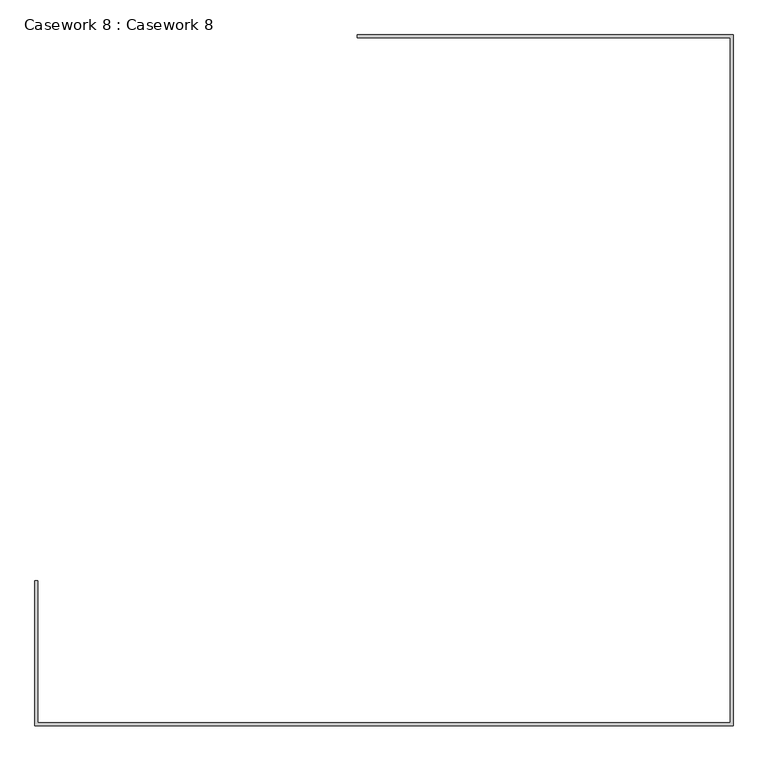
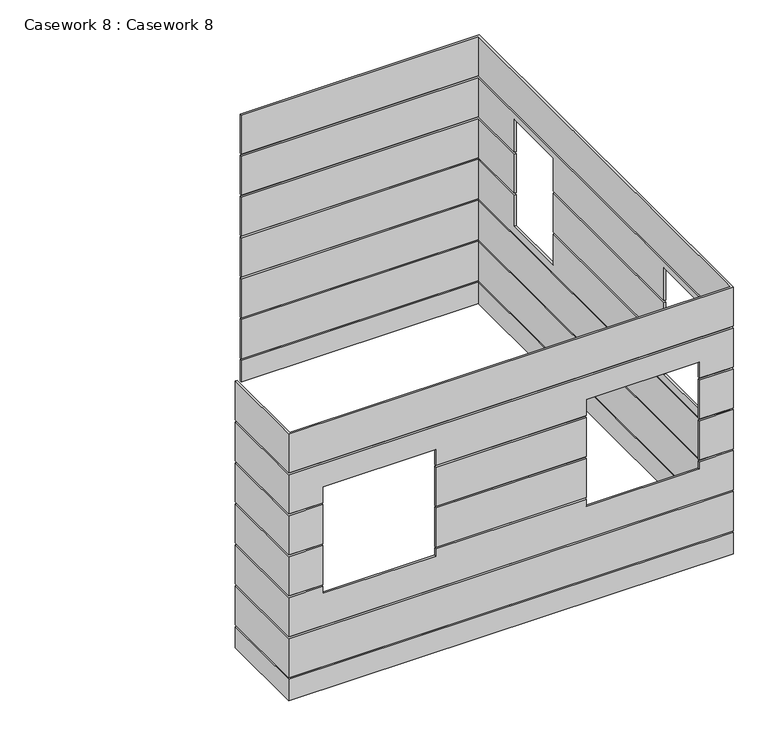
"""IFC4 building model written with IfcOpenShell, lengths in millimetres: furniture geometry, Casework 8 : Casework 8."""

from ifc_helpers import new_model, si_unit, origin, place, context, project, spatial, faceted_brep, source, transform, mapped, element, save


def casework_8_casework_8_de918fe4(model_context):
    return source(origin(), model_context, "Body", "Brep", [
        faceted_brep([(1963.2046034, -9896.6929163, 3750.0), (1988.2046034, -9896.6929163, 3750.0), (1988.2046034, -9896.6929163, 3200.0), (1963.2046034, -9896.6929163, 3200.0), (1963.2046034, -11121.6929163, 3750.0), (7863.2046034, -11121.6929163, 3750.0), (7863.2046034, -5284.1929163, 3750.0), (4688.2046034, -5284.1929163, 3750.0), (4688.2046034, -5309.1929163, 3750.0), (7838.2046034, -5309.1929163, 3750.0), (7838.2046034, -11096.6929163, 3750.0), (1988.2046034, -11096.6929163, 3750.0), (1988.2046034, -11096.6929163, 3200.0), (7838.2046034, -11096.6929163, 3200.0), (7838.2046034, -5309.1929163, 3200.0), (4688.2046034, -5309.1929163, 3200.0), (4688.2046034, -5284.1929163, 3200.0), (7863.2046034, -5284.1929163, 3200.0), (7863.2046034, -11121.6929163, 3200.0), (1963.2046034, -11121.6929163, 3200.0)], [[[0, 1, 2, 3]], [[1, 0, 4, 5, 6, 7, 8, 9, 10, 11]], [[2, 1, 11, 12]], [[3, 2, 12, 13, 14, 15, 16, 17, 18, 19]], [[0, 3, 19, 4]], [[11, 10, 13, 12]], [[5, 4, 19, 18]], [[10, 9, 14, 13]], [[6, 5, 18, 17]], [[8, 7, 16, 15]], [[9, 8, 15, 14]], [[7, 6, 17, 16]]]),
        faceted_brep([(1963.2046034, -9896.6929163, 3175.0), (1988.2046034, -9896.6929163, 3175.0), (1988.2046034, -9896.6929163, 2625.0), (1963.2046034, -9896.6929163, 2625.0), (1963.2046034, -11121.6929163, 3175.0), (7863.2046034, -11121.6929163, 3175.0), (7863.2046034, -5284.1929163, 3175.0), (4688.2046034, -5284.1929163, 3175.0), (4688.2046034, -5309.1929163, 3175.0), (7838.2046034, -5309.1929163, 3175.0), (7838.2046034, -11096.6929163, 3175.0), (1988.2046034, -11096.6929163, 3175.0), (1988.2046034, -11096.6929163, 2625.0), (2413.2046034, -11096.6929163, 2625.0), (2413.2046034, -11121.6929163, 2625.0), (1963.2046034, -11121.6929163, 2625.0), (7838.2046034, -5309.1929163, 2625.0), (4688.2046034, -5309.1929163, 2625.0), (4688.2046034, -5284.1929163, 2625.0), (7863.2046034, -5284.1929163, 2625.0), (7863.2046034, -6134.1929163, 2625.0), (7838.2046034, -6134.1929163, 2625.0), (7413.2046034, -11096.6929163, 2625.0), (7838.2046034, -11096.6929163, 2625.0), (7838.2046034, -10471.6929163, 2625.0), (7863.2046034, -10471.6929163, 2625.0), (7863.2046034, -11121.6929163, 2625.0), (7413.2046034, -11121.6929163, 2625.0), (3913.2046034, -11096.6929163, 2625.0), (5913.2046034, -11096.6929163, 2625.0), (5913.2046034, -11121.6929163, 2625.0), (3913.2046034, -11121.6929163, 2625.0), (7838.2046034, -9571.6929163, 2625.0), (7838.2046034, -7034.1929163, 2625.0), (7863.2046034, -7034.1929163, 2625.0), (7863.2046034, -9571.6929163, 2625.0), (7413.2046034, -11096.6929163, 2850.0), (5913.2046034, -11096.6929163, 2850.0), (3913.2046034, -11096.6929163, 2850.0), (2413.2046034, -11096.6929163, 2850.0), (2413.2046034, -11121.6929163, 2850.0), (3913.2046034, -11121.6929163, 2850.0), (5913.2046034, -11121.6929163, 2850.0), (7413.2046034, -11121.6929163, 2850.0), (7838.2046034, -6134.1929163, 3090.0), (7838.2046034, -7034.1929163, 3090.0), (7838.2046034, -9571.6929163, 3090.0), (7838.2046034, -10471.6929163, 3090.0), (7863.2046034, -10471.6929163, 3090.0), (7863.2046034, -9571.6929163, 3090.0), (7863.2046034, -7034.1929163, 3090.0), (7863.2046034, -6134.1929163, 3090.0)], [[[0, 1, 2, 3]], [[1, 0, 4, 5, 6, 7, 8, 9, 10, 11]], [[2, 1, 11, 12]], [[3, 2, 12, 13, 14, 15]], [[16, 17, 18, 19, 20, 21]], [[22, 23, 24, 25, 26, 27]], [[28, 29, 30, 31]], [[32, 33, 34, 35]], [[0, 3, 15, 4]], [[11, 10, 23, 22, 36, 37, 29, 28, 38, 39, 13, 12]], [[5, 4, 15, 14, 40, 41, 31, 30, 42, 43, 27, 26]], [[10, 9, 16, 21, 44, 45, 33, 32, 46, 47, 24, 23]], [[6, 5, 26, 25, 48, 49, 35, 34, 50, 51, 20, 19]], [[8, 7, 18, 17]], [[9, 8, 17, 16]], [[7, 6, 19, 18]], [[43, 36, 22, 27]], [[37, 42, 30, 29]], [[36, 43, 42, 37]], [[41, 38, 28, 31]], [[39, 40, 14, 13]], [[38, 41, 40, 39]], [[49, 46, 32, 35]], [[47, 48, 25, 24]], [[46, 49, 48, 47]], [[51, 44, 21, 20]], [[45, 50, 34, 33]], [[44, 51, 50, 45]]]),
        faceted_brep([(1963.2046034, -9896.6929163, 2600.0), (1988.2046034, -9896.6929163, 2600.0), (1988.2046034, -9896.6929163, 2050.0), (1963.2046034, -9896.6929163, 2050.0), (1963.2046034, -11121.6929163, 2600.0), (2413.2046034, -11121.6929163, 2600.0), (2413.2046034, -11096.6929163, 2600.0), (1988.2046034, -11096.6929163, 2600.0), (1988.2046034, -11096.6929163, 2050.0), (2413.2046034, -11096.6929163, 2050.0), (2413.2046034, -11121.6929163, 2050.0), (1963.2046034, -11121.6929163, 2050.0)], [[[0, 1, 2, 3]], [[1, 0, 4, 5, 6, 7]], [[2, 1, 7, 8]], [[3, 2, 8, 9, 10, 11]], [[0, 3, 11, 4]], [[8, 7, 6, 9]], [[4, 11, 10, 5]], [[6, 5, 10, 9]]]),
        faceted_brep([(1963.2046034, -9896.6929163, 2025.0), (1988.2046034, -9896.6929163, 2025.0), (1988.2046034, -9896.6929163, 1475.0), (1963.2046034, -9896.6929163, 1475.0), (1963.2046034, -11121.6929163, 2025.0), (2413.2046034, -11121.6929163, 2025.0), (2413.2046034, -11096.6929163, 2025.0), (1988.2046034, -11096.6929163, 2025.0), (1988.2046034, -11096.6929163, 1475.0), (2413.2046034, -11096.6929163, 1475.0), (2413.2046034, -11121.6929163, 1475.0), (1963.2046034, -11121.6929163, 1475.0)], [[[0, 1, 2, 3]], [[1, 0, 4, 5, 6, 7]], [[2, 1, 7, 8]], [[3, 2, 8, 9, 10, 11]], [[0, 3, 11, 4]], [[8, 7, 6, 9]], [[4, 11, 10, 5]], [[6, 5, 10, 9]]]),
        faceted_brep([(1963.2046034, -9896.6929163, 1450.0), (1988.2046034, -9896.6929163, 1450.0), (1988.2046034, -9896.6929163, 900.0), (1963.2046034, -9896.6929163, 900.0), (1963.2046034, -11121.6929163, 1450.0), (2413.2046034, -11121.6929163, 1450.0), (2413.2046034, -11096.6929163, 1450.0), (1988.2046034, -11096.6929163, 1450.0), (7863.2046034, -11121.6929163, 1450.0), (7863.2046034, -5284.1929163, 1450.0), (4688.2046034, -5284.1929163, 1450.0), (4688.2046034, -5309.1929163, 1450.0), (7838.2046034, -5309.1929163, 1450.0), (7838.2046034, -11096.6929163, 1450.0), (7413.2046034, -11096.6929163, 1450.0), (7413.2046034, -11121.6929163, 1450.0), (3913.2046034, -11121.6929163, 1450.0), (5913.2046034, -11121.6929163, 1450.0), (5913.2046034, -11096.6929163, 1450.0), (3913.2046034, -11096.6929163, 1450.0), (1988.2046034, -11096.6929163, 900.0), (7838.2046034, -11096.6929163, 900.0), (7838.2046034, -5309.1929163, 900.0), (4688.2046034, -5309.1929163, 900.0), (4688.2046034, -5284.1929163, 900.0), (7863.2046034, -5284.1929163, 900.0), (7863.2046034, -11121.6929163, 900.0), (1963.2046034, -11121.6929163, 900.0), (2413.2046034, -11096.6929163, 1350.0), (3913.2046034, -11096.6929163, 1350.0), (5913.2046034, -11096.6929163, 1350.0), (7413.2046034, -11096.6929163, 1350.0), (7413.2046034, -11121.6929163, 1350.0), (5913.2046034, -11121.6929163, 1350.0), (3913.2046034, -11121.6929163, 1350.0), (2413.2046034, -11121.6929163, 1350.0)], [[[0, 1, 2, 3]], [[1, 0, 4, 5, 6, 7]], [[8, 9, 10, 11, 12, 13, 14, 15]], [[16, 17, 18, 19]], [[2, 1, 7, 20]], [[3, 2, 20, 21, 22, 23, 24, 25, 26, 27]], [[0, 3, 27, 4]], [[20, 7, 6, 28, 29, 19, 18, 30, 31, 14, 13, 21]], [[27, 26, 8, 15, 32, 33, 17, 16, 34, 35, 5, 4]], [[13, 12, 22, 21]], [[9, 8, 26, 25]], [[11, 10, 24, 23]], [[12, 11, 23, 22]], [[10, 9, 25, 24]], [[31, 32, 15, 14]], [[32, 31, 30, 33]], [[33, 30, 18, 17]], [[29, 34, 16, 19]], [[34, 29, 28, 35]], [[35, 28, 6, 5]]]),
        faceted_brep([(1963.2046034, -9896.6929163, 875.0), (1988.2046034, -9896.6929163, 875.0), (1988.2046034, -9896.6929163, 325.0), (1963.2046034, -9896.6929163, 325.0), (1963.2046034, -11121.6929163, 875.0), (7863.2046034, -11121.6929163, 875.0), (7863.2046034, -5284.1929163, 875.0), (4688.2046034, -5284.1929163, 875.0), (4688.2046034, -5309.1929163, 875.0), (7838.2046034, -5309.1929163, 875.0), (7838.2046034, -11096.6929163, 875.0), (1988.2046034, -11096.6929163, 875.0), (1988.2046034, -11096.6929163, 325.0), (7838.2046034, -11096.6929163, 325.0), (7838.2046034, -5309.1929163, 325.0), (4688.2046034, -5309.1929163, 325.0), (4688.2046034, -5284.1929163, 325.0), (7863.2046034, -5284.1929163, 325.0), (7863.2046034, -11121.6929163, 325.0), (1963.2046034, -11121.6929163, 325.0)], [[[0, 1, 2, 3]], [[1, 0, 4, 5, 6, 7, 8, 9, 10, 11]], [[2, 1, 11, 12]], [[3, 2, 12, 13, 14, 15, 16, 17, 18, 19]], [[0, 3, 19, 4]], [[11, 10, 13, 12]], [[5, 4, 19, 18]], [[10, 9, 14, 13]], [[6, 5, 18, 17]], [[8, 7, 16, 15]], [[9, 8, 15, 14]], [[7, 6, 17, 16]]]),
        faceted_brep([(1963.2046034, -9896.6929163, 300.0), (1988.2046034, -9896.6929163, 300.0), (1988.2046034, -9896.6929163, 0.0), (1963.2046034, -9896.6929163, 0.0), (1963.2046034, -11121.6929163, 300.0), (7863.2046034, -11121.6929163, 300.0), (7863.2046034, -5284.1929163, 300.0), (4688.2046034, -5284.1929163, 300.0), (4688.2046034, -5309.1929163, 300.0), (7838.2046034, -5309.1929163, 300.0), (7838.2046034, -11096.6929163, 300.0), (1988.2046034, -11096.6929163, 300.0), (1988.2046034, -11096.6929163, 0.0), (7838.2046034, -11096.6929163, 0.0), (7838.2046034, -5309.1929163, 0.0), (4688.2046034, -5309.1929163, 0.0), (4688.2046034, -5284.1929163, 0.0), (7863.2046034, -5284.1929163, 0.0), (7863.2046034, -11121.6929163, 0.0), (1963.2046034, -11121.6929163, 0.0)], [[[0, 1, 2, 3]], [[1, 0, 4, 5, 6, 7, 8, 9, 10, 11]], [[2, 1, 11, 12]], [[3, 2, 12, 13, 14, 15, 16, 17, 18, 19]], [[0, 3, 19, 4]], [[11, 10, 13, 12]], [[5, 4, 19, 18]], [[10, 9, 14, 13]], [[6, 5, 18, 17]], [[8, 7, 16, 15]], [[9, 8, 15, 14]], [[7, 6, 17, 16]]]),
        faceted_brep([(7863.2046034, -5284.1929163, 2600.0), (4688.2046034, -5284.1929163, 2600.0), (4688.2046034, -5309.1929163, 2600.0), (7838.2046034, -5309.1929163, 2600.0), (7838.2046034, -6134.1929163, 2600.0), (7863.2046034, -6134.1929163, 2600.0), (7838.2046034, -5309.1929163, 2050.0), (4688.2046034, -5309.1929163, 2050.0), (4688.2046034, -5284.1929163, 2050.0), (7863.2046034, -5284.1929163, 2050.0), (7863.2046034, -6134.1929163, 2050.0), (7838.2046034, -6134.1929163, 2050.0)], [[[0, 1, 2, 3, 4, 5]], [[6, 7, 8, 9, 10, 11]], [[3, 6, 11, 4]], [[9, 0, 5, 10]], [[2, 1, 8, 7]], [[3, 2, 7, 6]], [[1, 0, 9, 8]], [[5, 4, 11, 10]]]),
        faceted_brep([(7413.2046034, -11121.6929163, 2600.0), (7863.2046034, -11121.6929163, 2600.0), (7863.2046034, -10471.6929163, 2600.0), (7838.2046034, -10471.6929163, 2600.0), (7838.2046034, -11096.6929163, 2600.0), (7413.2046034, -11096.6929163, 2600.0), (7413.2046034, -11096.6929163, 2050.0), (7838.2046034, -11096.6929163, 2050.0), (7838.2046034, -10471.6929163, 2050.0), (7863.2046034, -10471.6929163, 2050.0), (7863.2046034, -11121.6929163, 2050.0), (7413.2046034, -11121.6929163, 2050.0)], [[[0, 1, 2, 3, 4, 5]], [[6, 7, 8, 9, 10, 11]], [[4, 7, 6, 5]], [[10, 1, 0, 11]], [[7, 4, 3, 8]], [[1, 10, 9, 2]], [[0, 5, 6, 11]], [[3, 2, 9, 8]]]),
        faceted_brep([(3913.2046034, -11121.6929163, 2600.0), (5913.2046034, -11121.6929163, 2600.0), (5913.2046034, -11096.6929163, 2600.0), (3913.2046034, -11096.6929163, 2600.0), (3913.2046034, -11096.6929163, 2050.0), (5913.2046034, -11096.6929163, 2050.0), (5913.2046034, -11121.6929163, 2050.0), (3913.2046034, -11121.6929163, 2050.0)], [[[0, 1, 2, 3]], [[4, 5, 6, 7]], [[5, 4, 3, 2]], [[1, 0, 7, 6]], [[2, 1, 6, 5]], [[0, 3, 4, 7]]]),
        faceted_brep([(7863.2046034, -9571.6929163, 2600.0), (7863.2046034, -7034.1929163, 2600.0), (7838.2046034, -7034.1929163, 2600.0), (7838.2046034, -9571.6929163, 2600.0), (7838.2046034, -9571.6929163, 2050.0), (7838.2046034, -7034.1929163, 2050.0), (7863.2046034, -7034.1929163, 2050.0), (7863.2046034, -9571.6929163, 2050.0)], [[[0, 1, 2, 3]], [[4, 5, 6, 7]], [[5, 4, 3, 2]], [[1, 0, 7, 6]], [[0, 3, 4, 7]], [[2, 1, 6, 5]]]),
        faceted_brep([(7863.2046034, -5284.1929163, 2025.0), (4688.2046034, -5284.1929163, 2025.0), (4688.2046034, -5309.1929163, 2025.0), (7838.2046034, -5309.1929163, 2025.0), (7838.2046034, -6134.1929163, 2025.0), (7863.2046034, -6134.1929163, 2025.0), (7413.2046034, -11121.6929163, 2025.0), (7863.2046034, -11121.6929163, 2025.0), (7863.2046034, -10471.6929163, 2025.0), (7838.2046034, -10471.6929163, 2025.0), (7838.2046034, -11096.6929163, 2025.0), (7413.2046034, -11096.6929163, 2025.0), (7863.2046034, -9571.6929163, 2025.0), (7863.2046034, -7034.1929163, 2025.0), (7838.2046034, -7034.1929163, 2025.0), (7838.2046034, -9571.6929163, 2025.0), (7838.2046034, -11096.6929163, 1475.0), (7838.2046034, -5309.1929163, 1475.0), (4688.2046034, -5309.1929163, 1475.0), (4688.2046034, -5284.1929163, 1475.0), (7863.2046034, -5284.1929163, 1475.0), (7863.2046034, -11121.6929163, 1475.0), (7413.2046034, -11121.6929163, 1475.0), (7413.2046034, -11096.6929163, 1475.0), (7838.2046034, -10471.6929163, 1590.0), (7838.2046034, -9571.6929163, 1590.0), (7838.2046034, -7034.1929163, 1590.0), (7838.2046034, -6134.1929163, 1590.0), (7863.2046034, -6134.1929163, 1590.0), (7863.2046034, -7034.1929163, 1590.0), (7863.2046034, -9571.6929163, 1590.0), (7863.2046034, -10471.6929163, 1590.0)], [[[0, 1, 2, 3, 4, 5]], [[6, 7, 8, 9, 10, 11]], [[12, 13, 14, 15]], [[16, 17, 18, 19, 20, 21, 22, 23]], [[10, 16, 23, 11]], [[21, 7, 6, 22]], [[17, 16, 10, 9, 24, 25, 15, 14, 26, 27, 4, 3]], [[21, 20, 0, 5, 28, 29, 13, 12, 30, 31, 8, 7]], [[2, 1, 19, 18]], [[3, 2, 18, 17]], [[1, 0, 20, 19]], [[6, 11, 23, 22]], [[25, 30, 12, 15]], [[30, 25, 24, 31]], [[31, 24, 9, 8]], [[27, 28, 5, 4]], [[28, 27, 26, 29]], [[29, 26, 14, 13]]]),
        faceted_brep([(3913.2046034, -11121.6929163, 2025.0), (5913.2046034, -11121.6929163, 2025.0), (5913.2046034, -11096.6929163, 2025.0), (3913.2046034, -11096.6929163, 2025.0), (3913.2046034, -11096.6929163, 1475.0), (5913.2046034, -11096.6929163, 1475.0), (5913.2046034, -11121.6929163, 1475.0), (3913.2046034, -11121.6929163, 1475.0)], [[[0, 1, 2, 3]], [[4, 5, 6, 7]], [[5, 4, 3, 2]], [[1, 0, 7, 6]], [[2, 1, 6, 5]], [[0, 3, 4, 7]]]),
    ])


if __name__ == "__main__":
    model = new_model("IFC4")
    model_context = context("Model", 3, world=origin())
    ifc_project = project(units=[si_unit("LENGTHUNIT", "METRE", prefix="MILLI")], contexts=[model_context])
    site = spatial("IfcSite", under=ifc_project)
    building = spatial("IfcBuilding", under=site)
    placement = place(None, origin())
    casework_8_casework_8_shape = casework_8_casework_8_de918fe4(model_context)
    element("IfcFurniture", 1, ObjectType="Casework 8 : Casework 8", at=placement, inside=building, context=model_context, shape_type="MappedRepresentation", body=[
        mapped(casework_8_casework_8_shape, transform((0.0, 0.0, 0.0), x_axis=(1.0, 0.0, 0.0), y_axis=(0.0, 1.0, 0.0), z_axis=(0.0, 0.0, 1.0))),
    ])
    save(model, "model.ifc")
